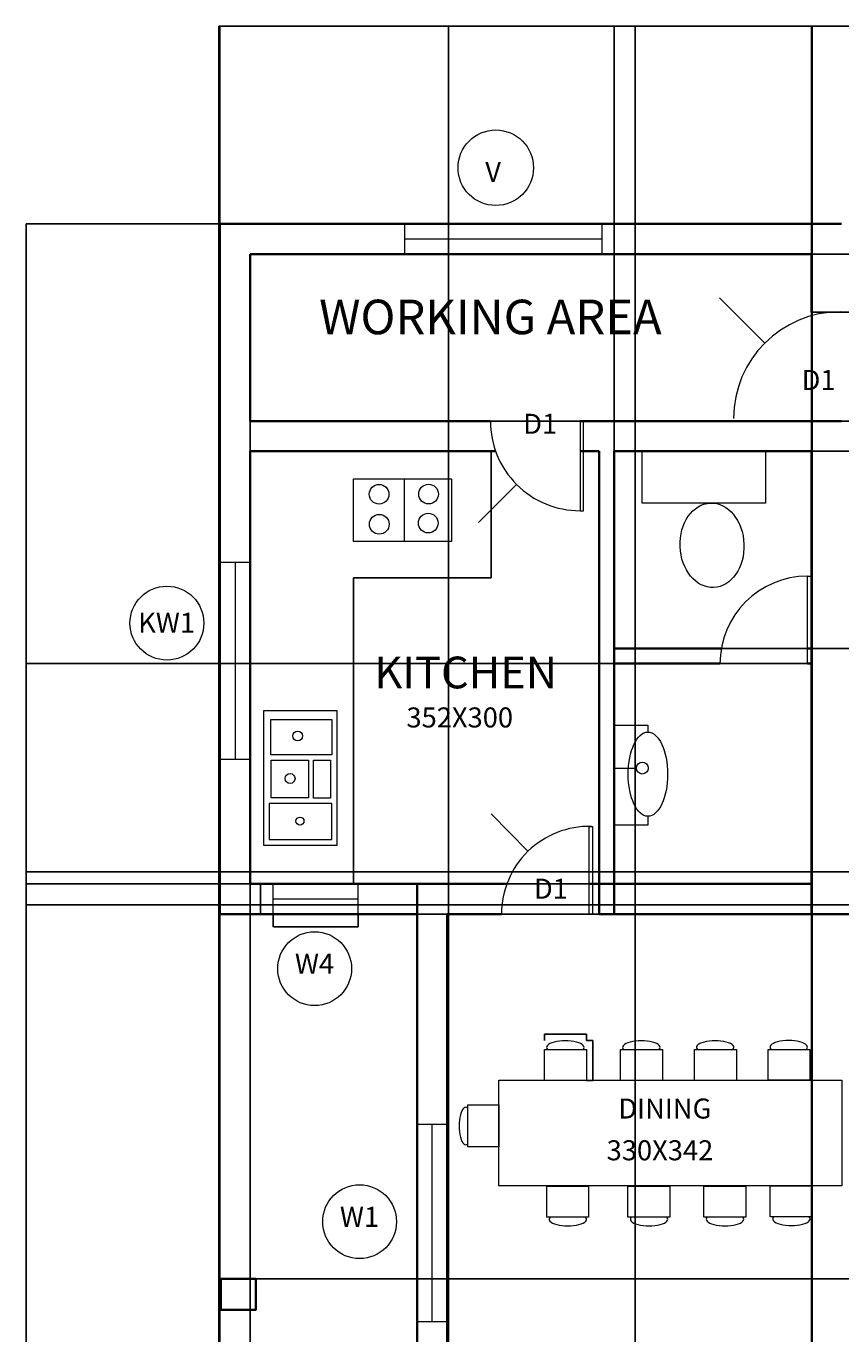
# Model space of a CAD drawing. Units: millimetres. Extents: x -2968 to 14333, y -2966 to 13411.
# Tile 2 of 3: x -2968 to 3229, y 3466 to 13411. Entities that reach past the tile are written whole.
import ezdxf

# ---------------------------------------------------------------- set-up
doc = ezdxf.new("R2010")
doc.units = ezdxf.units.MM
doc.header["$MEASUREMENT"] = 0
for name, color, linetype, lineweight in [('A-ANNO-DIMS', 2, 'Continuous', 18), ('A-ANNO-SYMB', 3, 'Continuous', 13), ('A-AREA-IDEN', 7, 'Continuous', 18), ('A-COLS', 7, 'Continuous', 35), ('A-DOOR', 3, 'Continuous', 18), ('A-EQPM', 8, 'Continuous', 18), ('A-FLOR-CASE', 8, 'Continuous', 25), ('A-FLOR-EDGE', 7, 'Continuous', 25), ('A-FLOR-FIXT', 9, 'Continuous', 18), ('A-FURN', 8, 'Continuous', 18), ('A-GLAZ', 4, 'Continuous', 18), ('A-WALL', 7, 'Continuous', 35)]:
    doc.layers.add(name, color=color, linetype=linetype, lineweight=lineweight)
doc.styles.get("Standard").update_dxf_attribs({"font": 'arial.ttf'})
doc.dimstyles.get("Standard").update_dxf_attribs({"dimtxt": 0.18, "dimasz": 0.18, "dimexe": 0.18, "dimexo": 0.0625, "dimgap": 0.09, "dimtad": 0, "dimtih": 1, "dimtoh": 1, "dimdec": 4, "dimzin": 0, "dimdsep": 46, "dimtxsty": 'Standard', "dimcen": 0.09, "dimadec": 0, "dimazin": 0, "dimtfac": 1, "dimtdec": 4, "dimtofl": 0, "dimtmove": 0, "dimatfit": 3, "dimfxl": 1, "dimtolj": 1, "dimtzin": 0, "dimarcsym": 0})

# ---------------------------------------------------------------- blocks, each defined once
blk = doc.blocks.new('DOOR-SWING-666')
blk.add_lwpolyline([(666.2992070210612, -7.87249337009e-05), (666.2992070210612, 666.0645318323222), (692.9797223629398, 666.0645318323222), (692.9797223629398, -7.87249337009e-05)], close=True)
blk.add_arc((666.2992070210612, -7.87249337009e-05), 666.2995763929106, 90, 180)
blk = doc.blocks.new('WIN-1500')
for p, q in [((-0.0001454069465439, 230.0001364428754), (-0.0001454069465439, 0.0001364428753732)), ((1499.999854593053, 230.0001364428754), (1499.999854593053, 0.0001364428753732)), ((-0.0001454069465439, 115.0001364428753), (1499.999854593053, 115.0001364428753))]:
    blk.add_line(p, q)
blk = doc.blocks.new('WIN-645')
for p, q in [((-0.0001783325678844, 645.3165217330161), (229.9998216674321, 645.3165217330161)), ((114.9998216674321, 645.3165217330161), (114.9998216674321, 9.39247611313e-05)), ((-0.0001783325678844, 9.39247611313e-05), (229.9998216674321, 9.39247611313e-05))]:
    blk.add_line(p, q)
blk = doc.blocks.new('DINING-CHAIR')
blk.add_lwpolyline([(8.40971169964e-05, 318.4642751495176), (234.8798944680875, 318.4642751495176), (234.8798944680875, -0.0002547686981416), (8.40971169964e-05, -0.0002547686981416)], close=True)
blk.add_ellipse((251.6572223520761, 161.1385219065178), major_axis=(0, 142.4711695614969), ratio=0.3529417904011299, start_param=2.801418553469442, end_param=6.623359407299936)
blk = doc.blocks.new('WC-PLAN')
blk.add_lwpolyline([(642.4076574105184, 937.925733504826), (1037.697987841055, 937.925733504826), (1037.697987841055, -0.0002773242667899), (642.4076574105184, -0.0002773242667899)], close=True)
blk.add_ellipse((321.2351413435845, 407.2568367539133), major_axis=(321.1725160669339, 12.34114489481309), ratio=0.7569293268408676)
blk = doc.blocks.new('VERANDAH-POST')
blk.add_lwpolyline([(-5.84108229305e-05, 235.3216454025205), (266.2404368537072, 235.3216454025205), (266.2404368537072, -0.0003482651118247), (-5.84108229305e-05, -0.0003482651118247)], close=True)
blk = doc.blocks.new('TAG-V')
blk.add_circle((287.0007825742364, 287.0011250592761), 287.0011736728098)
blk.add_text('V', height=152.3112078732942).set_placement((207.0741385544538, 179.2396726004772))
blk = doc.blocks.new('TAG-W1')
blk.add_circle((280.793431040287, 280.7932079668344), 280.7929963504647)
blk.add_text('W1', height=152.3112078732942).set_placement((130.9915239926576, 241.6268535788358))
blk = doc.blocks.new('TAG-W4')
blk.add_circle((280.792632550478, 280.7926029835935), 280.7929963504647)
blk.add_text('W4', height=152.3112078732942).set_placement((130.9907255028486, 241.6262485955949))
blk = doc.blocks.new('*D18')
at = {"layer": 'A-ANNO-DIMS', "color": 0, "lineweight": -2, "transparency": 16777216}
for p, q in [((-1087.823514483869, 6657.753456536686), (-1087.823514483869, 6560.838492365448)), ((-442.5070866756144, 6657.753456536685), (-442.5070866756147, 6560.838492365445)), ((-1087.643514483869, 6561.018492365448), (-766.353595259142, 6561.018492365447)), ((-442.6870866756147, 6561.018492365445), (-763.9770059003425, 6561.018492365447))]:
    blk.add_line(p, q, dxfattribs=at)
at = {"layer": 'A-ANNO-DIMS', "color": 0, "transparency": 16777216}
for points in [[(-1087.643514483869, 6561.048492365448), (-1087.643514483869, 6560.988492365448), (-1087.823514483869, 6561.018492365448)], [(-442.6870866756147, 6561.048492365445), (-442.6870866756147, 6560.988492365446), (-442.5070866756147, 6561.018492365445)]]:
    blk.add_solid(points, dxfattribs=at)
at = {"layer": 'Defpoints', "color": 0, "transparency": 16777216}
for p in [(-1087.823514483869, 6657.815956536686), (-442.5070866756144, 6657.815956536684), (-1087.823514483869, 6561.018492365448)]:
    blk.add_point(p, dxfattribs=at)
at = {"layer": 'A-ANNO-DIMS', "color": 0, "transparency": 16777216, "insert": (-765.1653005797422, 6561.018492365447), "char_height": 0.18, "attachment_point": 5}
blk.add_mtext('\\A1;WINDOW 645 TYP.', dxfattribs=at)
blk = doc.blocks.new('*D19')
at = {"layer": 'A-ANNO-DIMS', "color": 0, "lineweight": -2, "transparency": 16777216}
for p, q in [((-1087.886014483869, 6887.81595653669), (-1184.800978655108, 6887.81595653669)), ((-1184.620978655108, 6887.63595653669), (-1184.620978655108, 6772.997921066021)), ((-1184.620978655108, 6657.995956536691), (-1184.620978655108, 6772.633992007358)), ((-1087.88601448387, 6657.815956536691), (-1184.800978655108, 6657.815956536691))]:
    blk.add_line(p, q, dxfattribs=at)
at = {"layer": 'A-ANNO-DIMS', "color": 0, "transparency": 16777216}
for points in [[(-1184.650978655108, 6887.63595653669), (-1184.590978655108, 6887.63595653669), (-1184.620978655108, 6887.81595653669)], [(-1184.650978655108, 6657.995956536691), (-1184.590978655108, 6657.995956536691), (-1184.620978655108, 6657.815956536691)]]:
    blk.add_solid(points, dxfattribs=at)
at = {"layer": 'Defpoints', "color": 0, "transparency": 16777216}
for p in [(-1184.620978655108, 6887.81595653669), (-1087.823514483869, 6887.81595653669), (-1087.82351448387, 6657.815956536691)]:
    blk.add_point(p, dxfattribs=at)
at = {"layer": 'A-ANNO-DIMS', "color": 0, "transparency": 16777216, "insert": (-1184.620978655106, 6772.815956536688), "char_height": 0.18, "attachment_point": 5}
blk.add_mtext('\\A1;230 TYP.', dxfattribs=at)
blk = doc.blocks.new('*D24')
at = {"layer": 'A-ANNO-DIMS', "color": 0, "lineweight": -2, "transparency": 16777216}
for p, q in [((975.7055001648858, 5697.928340757243), (975.7055001648863, 5745.815520244975)), ((975.8855001648864, 5745.635520244975), (1133.443126651961, 5745.635520244974)), ((1293.990030083102, 5745.635520244972), (1136.432403596026, 5745.635520244974)), ((1294.170030083101, 5697.928340757241), (1294.170030083102, 5745.815520244972))]:
    blk.add_line(p, q, dxfattribs=at)
at = {"layer": 'A-ANNO-DIMS', "color": 0, "transparency": 16777216}
for points in [[(975.8855001648864, 5745.665520244974), (975.8855001648864, 5745.605520244975), (975.7055001648863, 5745.635520244975)], [(1293.990030083102, 5745.665520244973), (1293.990030083102, 5745.605520244972), (1294.170030083102, 5745.635520244972)]]:
    blk.add_solid(points, dxfattribs=at)
at = {"layer": 'Defpoints', "color": 0, "transparency": 16777216}
for p in [(975.7055001648863, 5745.635520244975), (975.7055001648858, 5697.865840757244), (1294.170030083101, 5697.865840757241)]:
    blk.add_point(p, dxfattribs=at)
at = {"layer": 'A-ANNO-DIMS', "color": 0, "transparency": 16777216, "insert": (1134.937765123994, 5745.635520244974), "char_height": 0.18, "attachment_point": 5}
blk.add_mtext('\\A1;DINING CHAIR 318 TYP.', dxfattribs=at)
blk = doc.blocks.new('*D25')
at = {"layer": 'A-ANNO-DIMS', "color": 0, "lineweight": -2, "transparency": 16777216}
for p, q in [((1294.232530083102, 5697.865840757243), (1342.119709570833, 5697.865840757243)), ((1341.939709570833, 5697.685840757243), (1341.939709570834, 5545.433684424839)), ((1341.939709570834, 5392.817599033771), (1341.939709570834, 5545.069755366176)), ((1294.232530083099, 5392.637599033771), (1342.119709570833, 5392.637599033771))]:
    blk.add_line(p, q, dxfattribs=at)
at = {"layer": 'A-ANNO-DIMS', "color": 0, "transparency": 16777216}
for points in [[(1341.909709570833, 5697.685840757243), (1341.969709570833, 5697.685840757243), (1341.939709570833, 5697.865840757243)], [(1341.909709570834, 5392.817599033771), (1341.969709570834, 5392.817599033771), (1341.939709570834, 5392.637599033771)]]:
    blk.add_solid(points, dxfattribs=at)
at = {"layer": 'Defpoints', "color": 0, "transparency": 16777216}
for p in [(1294.170030083102, 5697.865840757243), (1341.939709570833, 5697.865840757243), (1294.1700300831, 5392.637599033771)]:
    blk.add_point(p, dxfattribs=at)
at = {"layer": 'A-ANNO-DIMS', "color": 0, "transparency": 16777216, "insert": (1341.939709570835, 5545.251719895507), "char_height": 0.18, "attachment_point": 5}
blk.add_mtext('\\A1;305 TYP.', dxfattribs=at)
blk = doc.blocks.new('*D32')
at = {"layer": 'A-ANNO-DIMS', "color": 0, "lineweight": -2, "transparency": 16777216}
for p, q in [((-1494.810979, 11907.569973), (-1494.810979, 13410.507299)), ((-1494.630979, 13410.327299), (5659.769102855388, 13410.327299)), ((12815.009021, 13410.327299), (5660.608939144611, 13410.327299)), ((12815.189021, 11235.596939), (12815.189021, 13410.507299))]:
    blk.add_line(p, q, dxfattribs=at)
at = {"layer": 'A-ANNO-DIMS', "color": 0, "transparency": 16777216}
for points in [[(-1494.630979, 13410.357299), (-1494.630979, 13410.297299), (-1494.810979, 13410.327299)], [(12815.009021, 13410.357299), (12815.009021, 13410.297299), (12815.189021, 13410.327299)]]:
    blk.add_solid(points, dxfattribs=at)
at = {"layer": 'Defpoints', "color": 0, "transparency": 16777216}
for p in [(12815.189021, 13410.327299), (-1494.810979, 11907.507473), (12815.189021, 11235.534439)]:
    blk.add_point(p, dxfattribs=at)
at = {"layer": 'A-ANNO-DIMS', "color": 0, "transparency": 16777216, "insert": (5660.189021, 13410.327299), "char_height": 0.18, "attachment_point": 5}
blk.add_mtext('\\A1;14310', dxfattribs=at)
blk = doc.blocks.new('*D33')
at = {"layer": 'A-ANNO-DIMS', "color": 0, "lineweight": -2, "transparency": 16777216}
for p, q in [((-1494.873479, 11907.507473), (-2967.835419000003, 11907.507473)), ((-2967.655419000003, 11907.327473), (-2967.655419000002, 5205.189437529332)), ((-2967.655419, -1497.312527000001), (-2967.655419000002, 5204.825508470669)), ((-1494.873479, -1497.492527), (-2967.835419, -1497.492527000001))]:
    blk.add_line(p, q, dxfattribs=at)
at = {"layer": 'A-ANNO-DIMS', "color": 0, "transparency": 16777216}
for points in [[(-2967.685419000004, 11907.327473), (-2967.625419000004, 11907.327473), (-2967.655419000003, 11907.507473)], [(-2967.685419, -1497.312527000001), (-2967.625419, -1497.312527000001), (-2967.655419, -1497.492527000001)]]:
    blk.add_solid(points, dxfattribs=at)
at = {"layer": 'Defpoints', "color": 0, "transparency": 16777216}
for p in [(-2967.655419000003, 11907.507473), (-1494.810979, 11907.507473), (-1494.810979, -1497.492527)]:
    blk.add_point(p, dxfattribs=at)
at = {"layer": 'A-ANNO-DIMS', "color": 0, "transparency": 16777216, "insert": (-2967.655419, 5205.007473000001), "char_height": 0.18, "attachment_point": 5}
blk.add_mtext('\\A1;13405', dxfattribs=at)
blk = doc.blocks.new('*D45')
at = {"layer": 'A-ANNO-DIMS', "color": 0, "lineweight": -2, "transparency": 16777216}
for p, q in [((6467.303493000004, 6978.372882000003), (-2967.835419000002, 6978.372882000002)), ((-2967.655419000002, 6978.192882000001), (-2967.655419000002, 6853.554785137792)), ((-2967.655419000002, 6728.552882000002), (-2967.655419000002, 6853.190978862212)), ((6467.303493000004, 6728.372882000003), (-2967.835419000002, 6728.372882000002))]:
    blk.add_line(p, q, dxfattribs=at)
at = {"layer": 'A-ANNO-DIMS', "color": 0, "transparency": 16777216}
for points in [[(-2967.685419000002, 6978.192882000001), (-2967.625419000002, 6978.192882000001), (-2967.655419000002, 6978.372882000002)], [(-2967.685419000002, 6728.552882000002), (-2967.625419000002, 6728.552882000002), (-2967.655419000002, 6728.372882000002)]]:
    blk.add_solid(points, dxfattribs=at)
at = {"layer": 'Defpoints', "color": 0, "transparency": 16777216}
for p in [(-2967.655419000002, 6978.372882000002), (6467.365993000004, 6978.372882000003), (6467.365993000004, 6728.372882000003)]:
    blk.add_point(p, dxfattribs=at)
at = {"layer": 'A-ANNO-DIMS', "color": 0, "transparency": 16777216, "insert": (-2967.655419, 6853.372882000001), "char_height": 0.18, "attachment_point": 5}
blk.add_mtext('\\A1;250', dxfattribs=at)
blk = doc.blocks.new('*D46')
at = {"layer": 'A-ANNO-DIMS', "color": 0, "lineweight": -2, "transparency": 16777216}
for p, q in [((-1264.810979, 11677.444973), (-1264.810979000001, -2966.059788000001)), ((3005.189021, 11677.444973), (3005.189021, -2966.059788000001)), ((-1264.630979000001, -2965.879788), (869.8269336875846, -2965.879788)), ((3005.009020999999, -2965.879788), (870.551108312414, -2965.879788))]:
    blk.add_line(p, q, dxfattribs=at)
at = {"layer": 'A-ANNO-DIMS', "color": 0, "transparency": 16777216}
for points in [[(-1264.630979000001, -2965.849788), (-1264.630979000001, -2965.909788000001), (-1264.810979000001, -2965.879788)], [(3005.009020999999, -2965.849788), (3005.009020999999, -2965.909788000001), (3005.189021, -2965.879788)]]:
    blk.add_solid(points, dxfattribs=at)
at = {"layer": 'Defpoints', "color": 0, "transparency": 16777216}
for p in [(-1264.810979, 11677.507473), (3005.189021, 11677.507473), (3005.189021, -2965.879788)]:
    blk.add_point(p, dxfattribs=at)
at = {"layer": 'A-ANNO-DIMS', "color": 0, "transparency": 16777216, "insert": (870.1890209999993, -2965.879788), "char_height": 0.18, "attachment_point": 5}
blk.add_mtext('\\A1;4270', dxfattribs=at)
blk = doc.blocks.new('*D47')
at = {"layer": 'A-ANNO-DIMS', "color": 0, "lineweight": -2, "transparency": 16777216}
for p, q in [((-1264.748479, 11677.507473), (14333.28935600001, 11677.507473)), ((14333.10935600001, 11677.327473), (14333.10935600001, 11042.68937613779)), ((14333.10935600001, 10407.687473), (14333.10935600001, 11042.32556986221)), ((-1264.748479, 10407.507473), (14333.28935600001, 10407.507473))]:
    blk.add_line(p, q, dxfattribs=at)
at = {"layer": 'A-ANNO-DIMS', "color": 0, "transparency": 16777216}
for points in [[(14333.07935600001, 11677.327473), (14333.13935600001, 11677.327473), (14333.10935600001, 11677.507473)], [(14333.07935600001, 10407.687473), (14333.13935600001, 10407.687473), (14333.10935600001, 10407.507473)]]:
    blk.add_solid(points, dxfattribs=at)
at = {"layer": 'Defpoints', "color": 0, "transparency": 16777216}
for p in [(-1264.810979000001, 11677.507473), (14333.10935600001, 11677.507473), (-1264.810979000001, 10407.507473)]:
    blk.add_point(p, dxfattribs=at)
at = {"layer": 'A-ANNO-DIMS', "color": 0, "transparency": 16777216, "insert": (14333.10935600001, 11042.507473), "char_height": 0.18, "attachment_point": 5}
blk.add_mtext('\\A1;1270', dxfattribs=at)
blk = doc.blocks.new('*D54')
at = {"layer": 'A-ANNO-DIMS', "color": 0, "lineweight": -2, "transparency": 16777216}
for p, q in [((-1220.345468, 3884.149375000002), (14333.28935600001, 3884.149375000005)), ((14333.10935600001, 3883.969375000005), (14333.10935600001, 2738.596660637794)), ((14333.10935600001, 1592.860140000003), (14333.10935600001, 2738.232854362214)), ((-1220.345468, 1592.680140000001), (14333.28935600001, 1592.680140000003))]:
    blk.add_line(p, q, dxfattribs=at)
at = {"layer": 'A-ANNO-DIMS', "color": 0, "transparency": 16777216}
for points in [[(14333.07935600001, 3883.969375000005), (14333.13935600001, 3883.969375000005), (14333.10935600001, 3884.149375000005)], [(14333.07935600001, 1592.860140000003), (14333.13935600001, 1592.860140000003), (14333.10935600001, 1592.680140000003)]]:
    blk.add_solid(points, dxfattribs=at)
at = {"layer": 'Defpoints', "color": 0, "transparency": 16777216}
for p in [(-1220.407968, 3884.149375000002), (14333.10935600001, 3884.149375000005), (-1220.407968, 1592.680140000001)]:
    blk.add_point(p, dxfattribs=at)
at = {"layer": 'A-ANNO-DIMS', "color": 0, "transparency": 16777216, "insert": (14333.10935600001, 2738.414757499999), "char_height": 0.18, "attachment_point": 5}
blk.add_mtext('\\A1;2291.5', dxfattribs=at)
blk = doc.blocks.new('*D55')
at = {"layer": 'A-ANNO-DIMS', "color": 0, "lineweight": -2, "transparency": 16777216}
for p, q in [((-1494.748479, 6657.507473000004), (14333.28935600001, 6657.507473000006)), ((14333.10935600001, 6657.327473000005), (14333.10935600001, 5271.010388529336)), ((14333.10935600002, 3884.329375000005), (14333.10935600001, 5270.646459470672)), ((-1220.345468, 3884.149375000002), (14333.28935600002, 3884.149375000005))]:
    blk.add_line(p, q, dxfattribs=at)
at = {"layer": 'A-ANNO-DIMS', "color": 0, "transparency": 16777216}
for points in [[(14333.07935600001, 6657.327473000005), (14333.13935600001, 6657.327473000005), (14333.10935600001, 6657.507473000006)], [(14333.07935600002, 3884.329375000005), (14333.13935600001, 3884.329375000005), (14333.10935600002, 3884.149375000005)]]:
    blk.add_solid(points, dxfattribs=at)
at = {"layer": 'Defpoints', "color": 0, "transparency": 16777216}
for p in [(-1494.810979, 6657.507473000004), (14333.10935600001, 6657.507473000006), (-1220.407968, 3884.149375000002)]:
    blk.add_point(p, dxfattribs=at)
at = {"layer": 'A-ANNO-DIMS', "color": 0, "transparency": 16777216, "insert": (14333.10935600001, 5270.828424), "char_height": 0.18, "attachment_point": 5}
blk.add_mtext('\\A1;2773.4', dxfattribs=at)
blk = doc.blocks.new('*D56')
at = {"layer": 'A-ANNO-DIMS', "color": 0, "lineweight": -2, "transparency": 16777216}
for p, q in [((-1503.118196, -1242.758916), (-1503.118195999999, 13410.507299)), ((-1502.938195999999, 13410.327299), (80.61449804775, 13410.327299)), ((1664.884982000001, 13410.327299), (81.33228795225203, 13410.327299)), ((1665.064982, -1259.254558), (1665.064982000001, 13410.507299))]:
    blk.add_line(p, q, dxfattribs=at)
at = {"layer": 'A-ANNO-DIMS', "color": 0, "transparency": 16777216}
for points in [[(-1502.938195999999, 13410.357299), (-1502.938195999999, 13410.297299), (-1503.118195999999, 13410.327299)], [(1664.884982000001, 13410.357299), (1664.884982000001, 13410.297299), (1665.064982000001, 13410.327299)]]:
    blk.add_solid(points, dxfattribs=at)
at = {"layer": 'Defpoints', "color": 0, "transparency": 16777216}
for p in [(1665.064982000001, 13410.327299), (-1503.118196, -1242.821416), (1665.064982, -1259.317058)]:
    blk.add_point(p, dxfattribs=at)
at = {"layer": 'A-ANNO-DIMS', "color": 0, "transparency": 16777216, "insert": (80.97339300000101, 13410.327299), "char_height": 0.18, "attachment_point": 5}
blk.add_mtext('\\A1;3168', dxfattribs=at)
blk = doc.blocks.new('*D57')
at = {"layer": 'A-ANNO-DIMS', "color": 0, "lineweight": -2, "transparency": 16777216}
for p, q in [((1665.064982, -1259.254558), (1665.064982000001, 13410.507299)), ((1665.244982000001, 13410.327299), (3125.078715848568, 13410.327299)), ((4585.598316000001, 13410.327299), (3125.764582151433, 13410.327299)), ((4585.778315999999, -1259.254558), (4585.778316000001, 13410.507299))]:
    blk.add_line(p, q, dxfattribs=at)
at = {"layer": 'A-ANNO-DIMS', "color": 0, "transparency": 16777216}
for points in [[(1665.244982000001, 13410.357299), (1665.244982000001, 13410.297299), (1665.064982000001, 13410.327299)], [(4585.598316000001, 13410.357299), (4585.598316000001, 13410.297299), (4585.778316000001, 13410.327299)]]:
    blk.add_solid(points, dxfattribs=at)
at = {"layer": 'Defpoints', "color": 0, "transparency": 16777216}
for p in [(4585.778316000001, 13410.327299), (1665.064982, -1259.317058), (4585.778315999999, -1259.317058)]:
    blk.add_point(p, dxfattribs=at)
at = {"layer": 'A-ANNO-DIMS', "color": 0, "transparency": 16777216, "insert": (3125.421649000001, 13410.327299), "char_height": 0.18, "attachment_point": 5}
blk.add_mtext('\\A1;2921', dxfattribs=at)
blk = doc.blocks.new('*D58')
at = {"layer": 'A-ANNO-DIMS', "color": 0, "lineweight": -2, "transparency": 16777216}
for p, q in [((244.489985, 3229.006698), (244.4899850000006, 13410.507299)), ((244.6699850000006, 13410.327299), (1627.163433433834, 13410.327299)), ((3010.377373000001, 13410.327299), (1627.883924566167, 13410.327299)), ((3010.557373000001, 3229.006698), (3010.557373000001, 13410.507299))]:
    blk.add_line(p, q, dxfattribs=at)
at = {"layer": 'A-ANNO-DIMS', "color": 0, "transparency": 16777216}
for points in [[(244.6699850000006, 13410.357299), (244.6699850000006, 13410.297299), (244.4899850000006, 13410.327299)], [(3010.377373000001, 13410.357299), (3010.377373000001, 13410.297299), (3010.557373000001, 13410.327299)]]:
    blk.add_solid(points, dxfattribs=at)
at = {"layer": 'Defpoints', "color": 0, "transparency": 16777216}
for p in [(3010.557373000001, 13410.327299), (244.489985, 3228.944198), (3010.557373000001, 3228.944198)]:
    blk.add_point(p, dxfattribs=at)
at = {"layer": 'A-ANNO-DIMS', "color": 0, "transparency": 16777216, "insert": (1627.523679, 13410.327299), "char_height": 0.18, "attachment_point": 5}
blk.add_mtext('\\A1;2766', dxfattribs=at)
blk = doc.blocks.new('*D59')
at = {"layer": 'A-ANNO-DIMS', "color": 0, "lineweight": -2, "transparency": 16777216}
for p, q in [((1505.189021, 10177.569973), (1505.189021, 13410.507299)), ((1505.369021, 13410.327299), (2254.839027821283, 13410.327299)), ((3005.009021000001, 13410.327299), (2255.539014178718, 13410.327299)), ((3005.189021, 10177.569973), (3005.189021, 13410.507299))]:
    blk.add_line(p, q, dxfattribs=at)
at = {"layer": 'A-ANNO-DIMS', "color": 0, "transparency": 16777216}
for points in [[(1505.369021, 13410.357299), (1505.369021, 13410.297299), (1505.189021, 13410.327299)], [(3005.009021000001, 13410.357299), (3005.009021000001, 13410.297299), (3005.189021, 13410.327299)]]:
    blk.add_solid(points, dxfattribs=at)
at = {"layer": 'Defpoints', "color": 0, "transparency": 16777216}
for p in [(3005.189021, 13410.327299), (1505.189021, 10177.507473), (3005.189021, 10177.507473)]:
    blk.add_point(p, dxfattribs=at)
at = {"layer": 'A-ANNO-DIMS', "color": 0, "transparency": 16777216, "insert": (2255.189021, 13410.327299), "char_height": 0.18, "attachment_point": 5}
blk.add_mtext('\\A1;1500', dxfattribs=at)
blk = doc.blocks.new('*D60')
at = {"layer": 'A-ANNO-DIMS', "color": 0, "lineweight": -2, "transparency": 16777216}
for p, q in [((3005.126521000001, 8562.507473000003), (-2967.835419000003, 8562.507473000003)), ((-2967.655419000002, 8562.327473000003), (-2967.655419000002, 7725.189376137793)), ((-2967.655419000001, 6887.687473000003), (-2967.655419000002, 7724.825569862213)), ((3005.126521000001, 6887.507473000003), (-2967.835419000002, 6887.507473000002))]:
    blk.add_line(p, q, dxfattribs=at)
at = {"layer": 'A-ANNO-DIMS', "color": 0, "transparency": 16777216}
for points in [[(-2967.685419000002, 8562.327473000003), (-2967.625419000002, 8562.327473000003), (-2967.655419000002, 8562.507473000003)], [(-2967.685419000002, 6887.687473000003), (-2967.625419000001, 6887.687473000003), (-2967.655419000001, 6887.507473000002)]]:
    blk.add_solid(points, dxfattribs=at)
at = {"layer": 'Defpoints', "color": 0, "transparency": 16777216}
for p in [(-2967.655419000002, 8562.507473000003), (3005.189021000001, 8562.507473000003), (3005.189021000001, 6887.507473000003)]:
    blk.add_point(p, dxfattribs=at)
at = {"layer": 'A-ANNO-DIMS', "color": 0, "transparency": 16777216, "insert": (-2967.655419, 7725.007473000002), "char_height": 0.18, "attachment_point": 5}
blk.add_mtext('\\A1;1675', dxfattribs=at)
blk = doc.blocks.new('*D61')
at = {"layer": 'A-ANNO-DIMS', "color": 0, "lineweight": -2, "transparency": 16777216}
for p, q in [((1505.251521, 10177.507473), (14333.28935600001, 10177.507473)), ((14333.10935600001, 10177.327473), (14333.10935600001, 9427.689376137798)), ((14333.10935600001, 8677.687473000007), (14333.10935600001, 9427.325569862218)), ((1505.251521, 8677.507473000003), (14333.28935600001, 8677.507473000007))]:
    blk.add_line(p, q, dxfattribs=at)
at = {"layer": 'A-ANNO-DIMS', "color": 0, "transparency": 16777216}
for points in [[(14333.07935600001, 10177.327473), (14333.13935600001, 10177.327473), (14333.10935600001, 10177.507473)], [(14333.07935600001, 8677.687473000007), (14333.13935600001, 8677.687473000007), (14333.10935600001, 8677.507473000007)]]:
    blk.add_solid(points, dxfattribs=at)
at = {"layer": 'Defpoints', "color": 0, "transparency": 16777216}
for p in [(1505.189021, 10177.507473), (14333.10935600001, 10177.507473), (1505.189021, 8677.507473000003)]:
    blk.add_point(p, dxfattribs=at)
at = {"layer": 'A-ANNO-DIMS', "color": 0, "transparency": 16777216, "insert": (14333.10935600001, 9427.507473000001), "char_height": 0.18, "attachment_point": 5}
blk.add_mtext('\\A1;1500', dxfattribs=at)
blk = doc.blocks.new('*D65')
at = {"layer": 'A-ANNO-DIMS', "color": 0, "lineweight": -2, "transparency": 16777216}
for p, q in [((2306.527537003346, 11344.57574919665), (2306.707537003346, 11344.57574919665)), ((2306.707537003346, 11344.57574919665), (2650.618627832327, 11000.66437227355)), ((3224.053189999999, 10427.139333), (3224.233189999999, 10427.139333)), ((3224.143189999999, 10427.049333), (3224.143189999999, 10427.229333))]:
    blk.add_line(p, q, dxfattribs=at)
at = {"layer": 'A-ANNO-DIMS', "color": 0, "transparency": 16777216}
blk.add_solid([(2650.639841044587, 11000.68558546817), (2650.597414620067, 11000.64315907894), (2650.745907, 11000.537093)], dxfattribs=at)
at = {"layer": 'Defpoints', "color": 0, "transparency": 16777216}
for p in [(2650.745907, 11000.537093), (3224.143189999999, 10427.139333)]:
    blk.add_point(p, dxfattribs=at)
at = {"layer": 'A-ANNO-DIMS', "color": 0, "transparency": 16777216, "insert": (2306.047516539499, 11344.57574919665), "char_height": 0.18, "attachment_point": 5}
blk.add_mtext('\\A1;R810.9', dxfattribs=at)
blk = doc.blocks.new('*D66')
at = {"layer": 'A-ANNO-DIMS', "color": 0, "lineweight": -2, "transparency": 16777216}
for p, q in [((1244.927789999999, 10407.180857), (1245.10779, 10407.180857)), ((1245.017790000001, 10407.090857), (1245.017790000001, 10407.270857)), ((473.5450522253723, 9636.07761202546), (762.7200192958798, 9925.114080270192)), ((473.3650522253729, 9636.07761202546), (473.5450522253723, 9636.07761202546))]:
    blk.add_line(p, q, dxfattribs=at)
at = {"layer": 'A-ANNO-DIMS', "color": 0, "transparency": 16777216}
blk.add_solid([(762.6988111742457, 9925.135298554213), (762.741227417514, 9925.092861986173), (762.8473289999984, 9925.241329000002)], dxfattribs=at)
at = {"layer": 'Defpoints', "color": 0, "transparency": 16777216}
for p in [(1245.01779, 10407.180857), (762.8473289999984, 9925.241329000002)]:
    blk.add_point(p, dxfattribs=at)
at = {"layer": 'A-ANNO-DIMS', "color": 0, "transparency": 16777216, "insert": (472.6902977915387, 9636.07761202546), "char_height": 0.18, "attachment_point": 5}
blk.add_mtext('\\A1;2X R681.7', dxfattribs=at)
blk = doc.blocks.new('*D67')
at = {"layer": 'A-ANNO-DIMS', "color": 0, "lineweight": -2, "transparency": 16777216}
for p, q in [((569.6762104293579, 7421.685512974995), (569.8562104293587, 7421.685512974995)), ((569.8562104293587, 7421.685512974995), (848.8347249224774, 7135.589471172948)), ((1314.044025, 6658.419076), (1314.224025000001, 6658.419076000001)), ((1314.134025, 6658.329076), (1314.134025000001, 6658.509076))]:
    blk.add_line(p, q, dxfattribs=at)
at = {"layer": 'A-ANNO-DIMS', "color": 0, "transparency": 16777216}
blk.add_solid([(848.8562036179686, 7135.610415519201), (848.8132462269868, 7135.568526826694), (848.9603910000004, 7135.460598999999)], dxfattribs=at)
at = {"layer": 'Defpoints', "color": 0, "transparency": 16777216}
for p in [(848.9603910000004, 7135.460598999999), (1314.134025000001, 6658.419076)]:
    blk.add_point(p, dxfattribs=at)
at = {"layer": 'A-ANNO-DIMS', "color": 0, "transparency": 16777216, "insert": (569.0029907840653, 7421.685512974993), "char_height": 0.18, "attachment_point": 5}
blk.add_mtext('\\A1;5X R666.3', dxfattribs=at)

msp = doc.modelspace()

# ---------------------------------------------------------------- linework, layer by layer
at = {"layer": 'A-ANNO-SYMB'}
msp.add_circle((-1897.362422712147, 8870.842434626073), 280.7929963504647, dxfattribs=at)
at = {"layer": 'A-DOOR'}
msp.add_line((3224.143189993903, 11238.04588466449), (3224.143189993903, 11235.53443915362), dxfattribs=at)
for points in [[(1245.017790050479, 10407.18085732942), (1245.017790050479, 9725.6925334689), (1272.316132271152, 9725.6925334689), (1272.316132271152, 10407.18085732942)], [(1314.13402547325, 6658.419075832977), (1314.13402547325, 7324.483686390234), (1340.814540815128, 7324.483686390234), (1340.814540815128, 6658.419075832977)]]:
    msp.add_lwpolyline(points, close=True, dxfattribs=at)
for centre, radius, start, end in [((3224.143189993903, 10427.13933292603), 810.9065517384644, 90, 180), ((1245.017790050479, 10407.18085732942), 681.7287306783696, 179.9725496077652, 270), ((1314.13402547325, 6658.419075832977), 666.2995763929106, 88.47833873668723, 180.0783896496037)]:
    msp.add_arc(centre, radius, start, end, dxfattribs=at)
at = {"layer": 'A-EQPM'}
msp.add_line((-92.59458062052727, 9968.925373781472), (-92.59458062052727, 9492.387001253666), dxfattribs=at)
msp.add_lwpolyline([(-477.5140321478247, 9968.925373781472), (267.2569689154625, 9968.925373781472), (267.2569689154625, 9492.387001253666), (-477.5140321478247, 9492.387001253666)], close=True, dxfattribs=at)
for centre in [(-283.0258650407195, 9850.800167124718), (92.87156379222868, 9852.074045240879), (-281.8148552775383, 9622.322569455953), (90.26789281517267, 9631.369263220578)]:
    msp.add_circle(centre, 74.85653289780021, dxfattribs=at)
at = {"layer": 'A-FLOR-CASE'}
for points in [[(568.3745452016592, 9215.67476427555), (568.3745452016592, 10176.20045765862)], [(568.3745452016592, 9215.67476427555), (-477.2718301936984, 9215.67476427555), (-477.2718301936984, 6889.422179676592)]]:
    msp.add_lwpolyline(points, dxfattribs=at)
at = {"layer": 'A-FLOR-EDGE'}
for p, q in [((3005.189021442665, 11235.53443915362), (12815.18902144266, 11235.53443915362)), ((-1494.810978557335, 2.507473364634584), (-1494.810978557335, 6657.507473364635))]:
    msp.add_line(p, q, dxfattribs=at)
at = {"layer": 'A-FLOR-FIXT'}
for points in [[(-1163.551059961319, 7181.960732955485), (-601.4608808606863, 7181.960732955485), (-601.4608808606863, 8203.416664540768), (-1163.551059961319, 8203.416664540768)], [(-1106.936353780329, 8138.837521217764), (-643.1801670193672, 8138.837521217764), (-643.1801670193672, 7869.725370649248), (-1106.936353780329, 7869.725370649248)], [(-1103.484975971281, 7828.831723891198), (-820.4719955623149, 7828.831723891198), (-820.4719955623149, 7542.684152368456), (-1103.484975971281, 7542.684152368456)], [(-782.9912435635924, 7828.831723891198), (-653.4131994694471, 7828.831723891198), (-653.4131994694471, 7539.272749945522), (-782.9912435635924, 7539.272749945522)], [(-1120.560213558376, 7225.855550199748), (-643.1801670193672, 7225.855550199748), (-643.1801670193672, 7498.379103187471), (-1120.560213558376, 7498.379103187471)]]:
    msp.add_lwpolyline(points, close=True, dxfattribs=at)
for points in [[(1761.400808125734, 7401.767089237755), (1761.400808125734, 7335.042018860578), (1506.604355081916, 7335.042018860578), (1506.604355081916, 8095.33134475723), (1761.400808125734, 8095.33134475723), (1761.400808125734, 8042.57575138908)], [(1505.99885020405, 7768.095806084573), (1673.90535312891, 7768.095806084573)]]:
    msp.add_lwpolyline(points, dxfattribs=at)
for centre, radius in [((-902.3362551927567, 8012.788360834122), 37.54130248725414), ((1718.954916119576, 7768.095806084573), 45.04956299066543), ((-960.2830721065402, 7689.158544976264), 37.48224433511496), ((-885.2610176131129, 7365.528729114682), 30.65943949297071)]:
    msp.add_circle(centre, radius, dxfattribs=at)
msp.add_ellipse((1761.400808125734, 7722.171420313419), major_axis=(0, 320.4043310756623), ratio=0.4684851137277232, dxfattribs=at)
at = {"layer": 'A-FURN'}
msp.add_lwpolyline([(627.8926181816496, 5394.823160820234), (3236.742084097117, 5394.823160820234), (3236.742084097117, 4590.28017311683), (627.8926181816496, 4590.28017311683)], close=True, dxfattribs=at)
at = {"layer": 'A-WALL'}
for p, q in [((-1494.810978557335, 10407.50747336463), (-1494.810978557335, 11907.50747336463)), ((-1494.810978557335, 11907.50747336463), (3235.189021442665, 11907.50747336463)), ((-1264.810978557335, 10407.50747336463), (-1264.810978557335, 11677.50747336463)), ((-1264.810978557335, 11677.50747336463), (3005.189021442665, 11677.50747336463)), ((3005.189021442665, 11235.53443915362), (3005.189021442665, 11677.50747336463)), ((-1494.810978557335, 6657.507473364635), (-1494.810978557335, 10407.50747336463)), ((-1264.810978557335, 10407.50747336463), (563.2891376129369, 10407.50747336463)), ((1245.636054873233, 10407.50747336463), (3235.189021442665, 10407.50747336463)), ((-1264.810978557335, 10177.50747336463), (603.1422577776659, 10177.50747336464)), ((-1264.810978557335, 6887.507473364634), (-1264.810978557335, 10177.50747336463)), ((1245.017790050479, 10177.50747336463), (1390.189021442665, 10177.50747336463)), ((1390.189021442665, 6657.507473364635), (1390.189021442665, 10177.50747336463)), ((1505.189021442665, 6657.507473364635), (1505.189021442665, 10177.50747336463)), ((1505.189021442665, 10177.50747336463), (3005.189021442665, 10177.50747336463)), ((3005.189021442665, 6657.507473364635), (3005.189021442665, 10177.50747336463)), ((1505.189021442661, 8677.507473364638), (2319.569251334322, 8677.507473364636)), ((2975.712207021061, 8677.507473364634), (3005.189021442661, 8677.507473364634)), ((1505.189021442661, 8562.507473364638), (2309.413231126658, 8562.507473364636)), ((2975.712207021061, 8562.507473364634), (3005.189021442661, 8562.507473364634)), ((-1264.810978557335, 6887.507473364634), (688.4554885089801, 6887.507473364635)), ((5.189021442664909, 2.507473364634584), (5.189021442664909, 6887.507473364634)), ((1314.13402547325, 6887.507473364634), (3005.189021442665, 6887.507473364634)), ((-1494.810978557335, 6657.507473364635), (5.189021442664909, 6657.507473364635)), ((235.1890214426649, 1732.507473364634), (235.1890214426649, 6657.507473364635)), ((235.189021442665, 6657.507473364635), (647.8350726883068, 6657.507473364635)), ((1390.189021442665, 6657.507473364633), (6465.189021442665, 6657.507473364635))]:
    msp.add_line(p, q, dxfattribs=at)

# ---------------------------------------------------------------- block references
at = {"layer": 'A-ANNO-SYMB'}
for name, p in [('TAG-V', (317.038, 12046.825)), ('TAG-W4', (-1054.338, 5962.212)), ('TAG-W1', (-712.3496428769249, 4038.050881991985))]:
    msp.add_blockref(name, p, dxfattribs=at)
at = {"layer": 'A-COLS'}
msp.add_blockref('VERANDAH-POST', (-1486.648404935241, 3648.827729589135), dxfattribs=at)
at = {"layer": 'A-DOOR'}
msp.add_blockref('DOOR-SWING-666', (2309.413, 8561.613), dxfattribs=at)
at = {"layer": 'A-FLOR-FIXT', "rotation": 90.00000000000007}
msp.add_blockref('WC-PLAN', (2656.402211049883, 9141.416345577152), dxfattribs=at)
at = {"layer": 'A-FURN'}
for p, rotation in [((1294.169775314401, 5392.637514936652), 89.99999999999952), ((1872.694296823821, 5392.637514936652), 89.9999999999994), ((2434.202410051837, 5392.637514936652), 89.99999999999916), ((2993.889620253589, 5394.395084297199), 89.99999999999945), ((627.467692490055, 5207.179371439509), 180), ((991.4181325840696, 4589.204452279575), 269.9999999999997), ((1609.129599222441, 4589.204452279576), 269.9999999999996), ((2186.772859267186, 4589.204452279576), 269.9999999999995), ((2691.941398858783, 4590.823240077503), 270)]:
    msp.add_blockref('DINING-CHAIR', p, dxfattribs=dict(at, rotation=rotation))
at = {"layer": 'A-GLAZ'}
msp.add_blockref('WIN-1500', (-90.27, 11677.871), dxfattribs=at)
for name, p, rotation in [('WIN-1500', (-1493.310398346664, 9332.62250142176), 270), ('WIN-645', (-442.5069927508534, 6657.816134869252), 89.99999999999984), ('WIN-1500', (2.910328376419784, 5057.947653428108), 270)]:
    msp.add_blockref(name, p, dxfattribs=dict(at, rotation=rotation))

# ---------------------------------------------------------------- texts
at = {"layer": 'A-ANNO-SYMB'}
for s, p in [('D1', (2930.81238077581, 10643.9512302801)), ('D1', (813.0590667724609, 10310.23834523558)), ('KW1', (-2115.465280100703, 8797.562056016177)), ('D1', (894.7416749373077, 6774.924286991357))]:
    msp.add_text(s, height=152.3112078732942, dxfattribs=at).set_placement(p)
at = {"layer": 'A-AREA-IDEN'}
for s, height, p in [('WORKING AREA', 262.7143332324242, (-739.5535836826045, 11067.74951266594)), ('KITCHEN', 241.6627430388979, (-319.0630537954186, 8374.466654787433)), ('352X300', 152.3112078732942, (-75.3403804606296, 8077.259688549037)), ('DINING', 152.3112078732942, (1536.089753791084, 5103.164511058772)), ('330X342', 152.3112078732942, (1447.564940496673, 4785.623400789047))]:
    msp.add_text(s, height=height, dxfattribs=at).set_placement(p)

# ---------------------------------------------------------------- dimensions: what is measured, and where the dimension line sits
at = {"layer": 'A-ANNO-DIMS'}
for base, p1, p2, picture, middle in [((1665.064982000001, 13410.327299), (-1503.118196, -1242.821416), (1665.064982, -1259.317058), '*D56', (80.97339300000101, 13410.327299)), ((12815.189021, 13410.327299), (-1494.810979, 11907.507473), (12815.189021, 11235.534439), '*D32', (5660.189021, 13410.327299)), ((3010.557373000001, 13410.327299), (244.489985, 3228.944198), (3010.557373000001, 3228.944198), '*D58', (1627.523679, 13410.327299)), ((3005.189021, 13410.327299), (1505.189021, 10177.507473), (3005.189021, 10177.507473), '*D59', (2255.189021, 13410.327299)), ((4585.778316000001, 13410.327299), (1665.064982, -1259.317058), (4585.778315999999, -1259.317058), '*D57', (3125.421649000001, 13410.327299)), ((3005.189021, -2965.879788), (-1264.810979, 11677.507473), (3005.189021, 11677.507473), '*D46', (870.1890209999993, -2965.879788))]:
    dim = msp.add_linear_dim(base=base, p1=p1, p2=p2, dimstyle='Standard', override={"dimdec": 0, "dimlfac": 1, "dimrnd": 0, "dimzin": 0, "dimdsep": 46, "dimlunit": 2}, dxfattribs=at)
    dim.commit()
    dim.dimension.update_dxf_attribs({"geometry": picture, "text_midpoint": middle})
for base, p1, p2, override, picture, middle in [((-2967.655419000003, 11907.507473), (-1494.810979, -1497.492527), (-1494.810979, 11907.507473), {"dimdec": 0, "dimlfac": 1, "dimrnd": 0, "dimzin": 0, "dimdsep": 46, "dimlunit": 2}, '*D33', (-2967.655419, 5205.007473000001)), ((14333.10935600001, 11677.507473), (-1264.810979, 10407.507473), (-1264.810979, 11677.507473), {"dimdec": 0, "dimlfac": 1, "dimrnd": 0, "dimzin": 0, "dimdsep": 46, "dimlunit": 2}, '*D47', (14333.10935600001, 11042.507473)), ((14333.10935600001, 10177.507473), (1505.189021, 8677.507473), (1505.189021, 10177.507473), {"dimdec": 0, "dimlfac": 1, "dimrnd": 0, "dimzin": 0, "dimdsep": 46, "dimlunit": 2}, '*D61', (14333.10935600001, 9427.507473000001)), ((-2967.655419000002, 8562.507473000003), (3005.189021, 6887.507472999999), (3005.189021, 8562.507473), {"dimdec": 0, "dimlfac": 1, "dimrnd": 0, "dimzin": 0, "dimdsep": 46, "dimlunit": 2}, '*D60', (-2967.655419, 7725.007473000002)), ((-2967.655419000002, 6978.372882000002), (6467.365993, 6728.372881999999), (6467.365993, 6978.372881999999), {"dimdec": 0, "dimlfac": 1, "dimrnd": 0, "dimzin": 0, "dimdsep": 46, "dimlunit": 2}, '*D45', (-2967.655419, 6853.372882000001)), ((14333.10935600001, 6657.507473000006), (-1220.407968, 3884.149375), (-1494.810979, 6657.507472999999), {"dimdec": 1, "dimlfac": 1, "dimrnd": 0, "dimzin": 0, "dimdsep": 46, "dimlunit": 2}, '*D55', (14333.10935600001, 5270.828424)), ((14333.10935600001, 3884.149375000005), (-1220.407968, 1592.68014), (-1220.407968, 3884.149375), {"dimdec": 1, "dimlfac": 1, "dimrnd": 0, "dimzin": 0, "dimdsep": 46, "dimlunit": 2}, '*D54', (14333.10935600001, 2738.414757499999))]:
    dim = msp.add_linear_dim(base=base, p1=p1, p2=p2, angle=90, dimstyle='Standard', override=override, dxfattribs=at)
    dim.commit()
    dim.dimension.update_dxf_attribs({"geometry": picture, "text_midpoint": middle})
dim = msp.add_radius_dim(center=(3224.143189999999, 10427.139333), mpoint=(2650.745907, 11000.537093), dimstyle='Standard', override={"dimdec": 1, "dimlfac": 1, "dimrnd": 0, "dimzin": 0, "dimdsep": 46, "dimlunit": 2}, dxfattribs=at)
dim.commit()
dim.dimension.update_dxf_attribs({"geometry": '*D65', "text_midpoint": (2306.047516539499, 11344.57574919665), "dimtype": 164})
for center, mpoint, text, picture, middle in [((1245.01779, 10407.180857), (762.8473289999984, 9925.241329000002), '2X <>', '*D66', (472.6902977915387, 9636.07761202546)), ((1314.134025000001, 6658.419076), (848.9603910000004, 7135.460598999999), '5X <>', '*D67', (569.0029907840653, 7421.685512974993))]:
    dim = msp.add_radius_dim(center=center, mpoint=mpoint, text=text, dimstyle='Standard', override={"dimdec": 1, "dimlfac": 1, "dimrnd": 0, "dimzin": 0, "dimdsep": 46, "dimlunit": 2}, dxfattribs=at)
    dim.commit()
    dim.dimension.update_dxf_attribs({"geometry": picture, "text_midpoint": middle, "dimtype": 164})
for base, p1, p2, angle, text, picture, middle in [((-1184.620978655108, 6887.81595653669), (-1087.823514483869, 6657.815956536686), (-1087.823514483869, 6887.815956536686), 89.99999999999984, '<> TYP.', '*D19', (-1184.620978655106, 6772.815956536688)), ((-1087.823514483869, 6561.018492365448), (-442.5070866756144, 6657.815956536684), (-1087.823514483869, 6657.815956536686), 179.9999999999998, 'WINDOW <> TYP.', '*D18', (-765.1653005797422, 6561.018492365447)), ((975.7055001648863, 5745.635520244975), (1294.170030083101, 5697.865840757241), (975.7055001648858, 5697.865840757244), 179.9999999999995, 'DINING CHAIR <> TYP.', '*D24', (1134.937765123994, 5745.635520244974)), ((1341.939709570833, 5697.865840757243), (1294.170030083099, 5392.637599033769), (1294.170030083101, 5697.865840757241), 89.99999999999953, '<> TYP.', '*D25', (1341.939709570835, 5545.251719895507))]:
    dim = msp.add_linear_dim(base=base, p1=p1, p2=p2, angle=angle, text=text, dimstyle='Standard', override={"dimdec": 0, "dimlfac": 1, "dimrnd": 0, "dimzin": 0, "dimdsep": 46, "dimlunit": 2}, dxfattribs=at)
    dim.commit()
    dim.dimension.update_dxf_attribs({"geometry": picture, "text_midpoint": middle})

doc.saveas('drawing.dxf')
